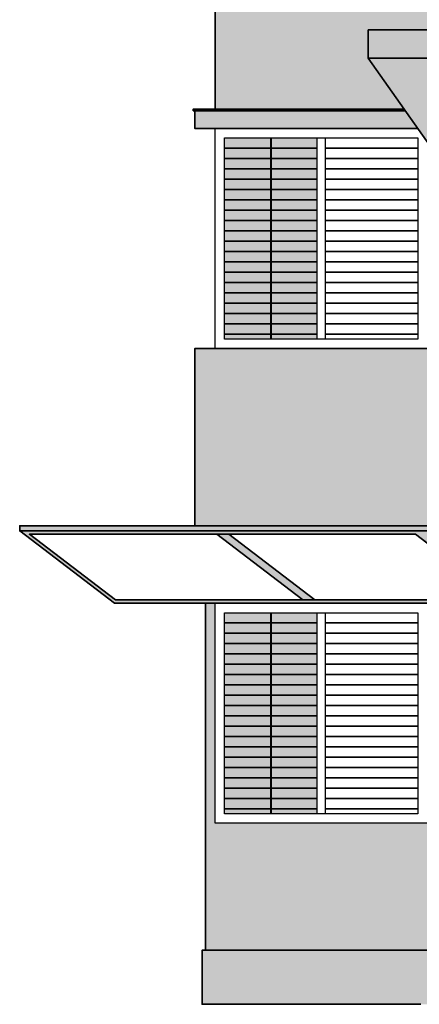
# Model space of a CAD drawing. Units: feet. Extents: x 2613 to 3913, y 950 to 1393.
# Tile 1 of 6: x 2613 to 2725, y 950 to 1226. Entities that reach past the tile are written whole.
import ezdxf

# ---------------------------------------------------------------- set-up
doc = ezdxf.new("R2010")
doc.units = ezdxf.units.FT
for name, color, linetype, lineweight in [('A-ELEV', 7, 'Continuous', 35), ('A-ELEV-PATT', 9, 'Continuous', 13), ('A-GLAZ', 4, 'Continuous', 25)]:
    doc.layers.add(name, color=color, linetype=linetype, lineweight=lineweight)

msp = doc.modelspace()

# ---------------------------------------------------------------- hatches: boundary and pattern name
at = {"layer": 'A-ELEV-PATT'}
h = msp.add_hatch(color=256, dxfattribs=at)
h.dxf.hatch_style = 1
h.paths.add_polyline_path([(3108.91, 1328.81), (3061.44, 1376.28), (2929.45, 1244.29), (2929.45, 1223.38), (2942.09, 1223.38), (2942.09, 1215.5), (2929.45, 1215.5), (2929.45, 1084.12), (3108.91, 1084.12), (3108.91, 1199.69), (3106.87, 1199.69), (3106.87, 1128.72), (3017.91, 1128.72), (3017.91, 1199.69), (3008.08, 1199.69), (3008.08, 1180.01), (3007.65, 1180.01), (3007.65, 1199.69), (3004.75, 1199.69), (3004.75, 1206.47), (3108.91, 1206.47)])
h.paths.add_polyline_path([(3061.44, 1376.28), (3193.8, 1243.92), (3193.8, 1233.84), (3204.34, 1246.9), (3061.54, 1389.71), (2918.82, 1247), (2929.45, 1233.69), (2929.45, 1244.29)])
h.paths.add_polyline_path([(3061.54, 1389.71), (3204.34, 1246.9), (3206.69, 1248.02), (3061.63, 1393.09), (2916.59, 1248.06), (2918.82, 1247)])
h.paths.add_polyline_path([(2925.65, 1257.12), (2667.59, 1257.12), (2651.33, 1257.12), (2651.33, 1252.28), (2920.82, 1252.28)])
h.paths.add_polyline_path([(2920.82, 1252.28), (2651.33, 1252.28, -0.144454), (2652.15, 1251.12), (2667.59, 1251.12), (2919.65, 1251.12)])
h.paths.add_polyline_path([(2918.82, 1247), (2916.59, 1248.06), (2919.65, 1251.12), (2667.59, 1251.12), (2652.15, 1251.12), (2667.59, 1229.14), (2667.59, 1233.69), (2929.45, 1233.69)])
h.paths.add_polyline_path([(2710.6, 1223.38), (2929.45, 1223.38), (2929.45, 1233.69), (2667.59, 1233.69), (2667.59, 1229.14), (2667.59, 1201.16), (2720.67, 1201.16), (2710.6, 1215.5)])
h.paths.add_polyline_path([(2942.09, 1223.38), (2710.6, 1223.38), (2710.6, 1215.5), (2921.48, 1215.5), (2942.09, 1215.5)])
h.paths.add_polyline_path([(2929.45, 1215.5), (2921.48, 1215.5), (2710.6, 1215.5), (2733.47, 1182.94), (2733.47, 1195.74), (2741.22, 1195.74), (2929.45, 1195.74)])
h.paths.add_polyline_path([(2721, 1200.68), (2661.89, 1200.68), (2661.89, 1195.74), (2724.47, 1195.74)])
h.paths.add_polyline_path([(2733.47, 1182.94), (2727.27, 1191.76), (2727.27, 1133.88), (2731.7, 1133.88), (2731.7, 1169.74), (2731.61, 1169.74), (2731.61, 1170.13), (2733.47, 1170.13)])
h.paths.add_polyline_path([(2929.45, 1183.04), (2741.22, 1183.04), (2741.22, 1170.13), (2743.07, 1170.13), (2743.07, 1169.74), (2743.07, 1112.32), (2759.57, 1112.32), (2759.57, 1167.82), (2763.7, 1167.82), (2763.7, 1112.32), (2781.75, 1112.32), (2781.75, 1167.82), (2785.87, 1167.82), (2785.87, 1112.32), (2803.92, 1112.32), (2803.92, 1167.82), (2808.05, 1167.82), (2808.05, 1112.32), (2826.09, 1112.32), (2826.09, 1167.82), (2830.22, 1167.82), (2830.22, 1112.32), (2875.17, 1112.32), (2875.17, 1171.49), (2929.45, 1171.49)])
h.paths.add_polyline_path([(2731.7, 1133.88), (2661.89, 1133.88), (2661.89, 1084.12), (2730.99, 1084.12), (2730.99, 1112.32), (2731.7, 1112.32)])
h.paths.add_polyline_path([(2929.45, 1112.32), (2730.99, 1112.32), (2730.99, 1084.12), (2929.45, 1084.12)])
h.paths.add_polyline_path([(2929.45, 1084.12), (2730.99, 1084.12), (2661.89, 1084.12), (2612.72, 1084.12), (2612.72, 1082.68), (2929.45, 1082.68)])
h.paths.add_polyline_path([(2929.45, 1082.68), (2612.72, 1082.68), (2639.32, 1062.44), (2733.47, 1062.44), (2733.47, 1063.35), (2639.62, 1063.35), (2615.43, 1081.77), (2723.91, 1081.77), (2739.71, 1069.74), (2741.22, 1069.74), (2725.42, 1081.77), (2929.45, 1081.77)])
h.paths.add_polyline_path([(2671.42, 1081.77), (2668.07, 1081.77), (2692.27, 1063.35), (2695.62, 1063.35)], flags=17)
h.paths.add_polyline_path([(2741.22, 1069.74), (2741.22, 1068.59), (2748.11, 1063.35), (2741.22, 1063.35), (2741.22, 1062.44), (2750.82, 1062.44)], flags=17)
h.paths.add_polyline_path([(2929.45, 1081.77), (2725.42, 1081.77), (2750.82, 1062.44), (2741.22, 1062.44), (2741.22, 1047.95), (2743.07, 1047.95), (2743.07, 1047.56), (2743.07, 967.97), (2875.17, 967.97), (2875.17, 1066.37), (2929.45, 1066.37)])
h.paths.add_polyline_path([(2778.55, 1066.37), (2806.94, 1066.37), (2806.94, 982.04), (2778.55, 982.04)], flags=16)
h.paths.add_polyline_path([(2778.55, 1064.05), (2806.94, 1064.05), (2806.94, 1063.39), (2778.55, 1063.39)], flags=16)
h.paths.add_polyline_path([(2778.55, 1061.07), (2806.94, 1061.07), (2806.94, 1060.41), (2778.55, 1060.41)], flags=0)
h.paths.add_polyline_path([(2778.55, 1058.09), (2806.94, 1058.09), (2806.94, 1057.43), (2778.55, 1057.43)], flags=0)
h.paths.add_polyline_path([(2778.55, 1055.11), (2806.94, 1055.11), (2806.94, 1054.45), (2778.55, 1054.45)], flags=0)
h.paths.add_polyline_path([(2778.55, 1052.13), (2806.94, 1052.13), (2806.94, 1051.47), (2778.55, 1051.47)], flags=0)
h.paths.add_polyline_path([(2778.55, 1049.15), (2806.94, 1049.15), (2806.94, 1048.49), (2778.55, 1048.49)], flags=0)
h.paths.add_polyline_path([(2778.55, 1046.18), (2806.94, 1046.18), (2806.94, 1045.51), (2778.55, 1045.51)], flags=0)
h.paths.add_polyline_path([(2778.55, 1043.2), (2806.94, 1043.2), (2806.94, 1042.53), (2778.55, 1042.53)], flags=0)
h.paths.add_polyline_path([(2778.55, 1040.22), (2806.94, 1040.22), (2806.94, 1039.56), (2778.55, 1039.56)], flags=0)
h.paths.add_polyline_path([(2778.55, 1037.24), (2806.94, 1037.24), (2806.94, 1036.58), (2778.55, 1036.58)], flags=0)
h.paths.add_polyline_path([(2778.55, 1034.26), (2806.94, 1034.26), (2806.94, 1033.6), (2778.55, 1033.6)], flags=0)
h.paths.add_polyline_path([(2778.55, 1031.28), (2806.94, 1031.28), (2806.94, 1030.62), (2778.55, 1030.62)], flags=0)
h.paths.add_polyline_path([(2778.55, 1028.3), (2806.94, 1028.3), (2806.94, 1027.64), (2778.55, 1027.64)], flags=0)
h.paths.add_polyline_path([(2778.55, 1025.32), (2806.94, 1025.32), (2806.94, 1024.66), (2778.55, 1024.66)], flags=0)
h.paths.add_polyline_path([(2778.55, 1022.34), (2806.94, 1022.34), (2806.94, 1021.68), (2778.55, 1021.68)], flags=0)
h.paths.add_polyline_path([(2778.55, 1019.36), (2806.94, 1019.36), (2806.94, 1018.7), (2778.55, 1018.7)], flags=0)
h.paths.add_polyline_path([(2778.55, 1016.71), (2806.94, 1016.71), (2806.94, 1016.05), (2778.55, 1016.05)], flags=0)
h.paths.add_polyline_path([(2824.02, 1066.37), (2852.41, 1066.37), (2852.41, 982.04), (2824.02, 982.04)], flags=16)
h.paths.add_polyline_path([(2778.55, 1014.07), (2806.94, 1014.07), (2806.94, 1013.4), (2778.55, 1013.4)], flags=0)
h.paths.add_polyline_path([(2824.02, 1064.05), (2852.41, 1064.05), (2852.41, 1063.39), (2824.02, 1063.39)], flags=16)
h.paths.add_polyline_path([(2824.02, 1061.07), (2852.41, 1061.07), (2852.41, 1060.41), (2824.02, 1060.41)], flags=0)
h.paths.add_polyline_path([(2824.02, 1058.09), (2852.41, 1058.09), (2852.41, 1057.43), (2824.02, 1057.43)], flags=0)
h.paths.add_polyline_path([(2824.02, 1055.11), (2852.41, 1055.11), (2852.41, 1054.45), (2824.02, 1054.45)], flags=16)
h.paths.add_polyline_path([(2824.02, 1052.13), (2852.41, 1052.13), (2852.41, 1051.47), (2824.02, 1051.47)], flags=0)
h.paths.add_polyline_path([(2778.55, 1011.09), (2806.94, 1011.09), (2806.94, 1010.43), (2778.55, 1010.43)], flags=0)
h.paths.add_polyline_path([(2824.02, 1049.15), (2852.41, 1049.15), (2852.41, 1048.49), (2824.02, 1048.49)], flags=0)
h.paths.add_polyline_path([(2824.02, 1046.18), (2852.41, 1046.18), (2852.41, 1045.51), (2824.02, 1045.51)], flags=0)
h.paths.add_polyline_path([(2824.02, 1043.2), (2852.41, 1043.2), (2852.41, 1042.53), (2824.02, 1042.53)], flags=0)
h.paths.add_polyline_path([(2778.55, 1008.11), (2806.94, 1008.11), (2806.94, 1007.45), (2778.55, 1007.45)], flags=0)
h.paths.add_polyline_path([(2824.02, 1040.22), (2852.41, 1040.22), (2852.41, 1039.56), (2824.02, 1039.56)], flags=0)
h.paths.add_polyline_path([(2824.02, 1037.24), (2852.41, 1037.24), (2852.41, 1036.58), (2824.02, 1036.58)], flags=0)
h.paths.add_polyline_path([(2778.55, 1005.13), (2806.94, 1005.13), (2806.94, 1004.47), (2778.55, 1004.47)], flags=0)
h.paths.add_polyline_path([(2824.02, 1034.26), (2852.41, 1034.26), (2852.41, 1033.6), (2824.02, 1033.6)], flags=0)
h.paths.add_polyline_path([(2824.02, 1031.28), (2852.41, 1031.28), (2852.41, 1030.62), (2824.02, 1030.62)], flags=0)
h.paths.add_polyline_path([(2778.55, 1002.15), (2806.94, 1002.15), (2806.94, 1001.49), (2778.55, 1001.49)], flags=0)
h.paths.add_polyline_path([(2824.02, 1028.3), (2852.41, 1028.3), (2852.41, 1027.64), (2824.02, 1027.64)], flags=0)
h.paths.add_polyline_path([(2778.55, 999.17), (2806.94, 999.17), (2806.94, 998.51), (2778.55, 998.51)], flags=0)
h.paths.add_polyline_path([(2824.02, 1025.32), (2852.41, 1025.32), (2852.41, 1024.66), (2824.02, 1024.66)], flags=0)
h.paths.add_polyline_path([(2824.02, 1022.34), (2852.41, 1022.34), (2852.41, 1021.68), (2824.02, 1021.68)], flags=0)
h.paths.add_polyline_path([(2778.55, 996.19), (2806.94, 996.19), (2806.94, 995.53), (2778.55, 995.53)], flags=0)
h.paths.add_polyline_path([(2824.02, 1019.36), (2852.41, 1019.36), (2852.41, 1018.7), (2824.02, 1018.7)], flags=0)
h.paths.add_polyline_path([(2778.55, 993.21), (2806.94, 993.21), (2806.94, 992.55), (2778.55, 992.55)], flags=0)
h.paths.add_polyline_path([(2824.02, 1016.38), (2852.41, 1016.38), (2852.41, 1015.72), (2824.02, 1015.72)], flags=0)
h.paths.add_polyline_path([(2824.02, 1013.4), (2852.41, 1013.4), (2852.41, 1012.74), (2824.02, 1012.74)], flags=0)
h.paths.add_polyline_path([(2778.55, 990.23), (2806.94, 990.23), (2806.94, 989.57), (2778.55, 989.57)], flags=0)
h.paths.add_polyline_path([(2824.02, 1010.43), (2852.41, 1010.43), (2852.41, 1009.76), (2824.02, 1009.76)], flags=0)
h.paths.add_polyline_path([(2778.55, 987.25), (2806.94, 987.25), (2806.94, 986.59), (2778.55, 986.59)], flags=0)
h.paths.add_polyline_path([(2824.02, 1007.45), (2852.41, 1007.45), (2852.41, 1006.78), (2824.02, 1006.78)], flags=0)
h.paths.add_polyline_path([(2778.55, 984.27), (2806.94, 984.27), (2806.94, 983.61), (2778.55, 983.61)], flags=0)
h.paths.add_polyline_path([(2824.02, 1004.47), (2852.41, 1004.47), (2852.41, 1003.81), (2824.02, 1003.81)], flags=0)
h.paths.add_polyline_path([(2824.02, 1001.49), (2852.41, 1001.49), (2852.41, 1000.83), (2824.02, 1000.83)], flags=0)
h.paths.add_polyline_path([(2824.02, 998.51), (2852.41, 998.51), (2852.41, 997.85), (2824.02, 997.85)], flags=0)
h.paths.add_polyline_path([(2824.02, 995.53), (2852.41, 995.53), (2852.41, 994.87), (2824.02, 994.87)], flags=0)
h.paths.add_polyline_path([(2824.02, 992.55), (2852.41, 992.55), (2852.41, 991.89), (2824.02, 991.89)], flags=0)
h.paths.add_polyline_path([(2824.02, 989.57), (2852.41, 989.57), (2852.41, 988.91), (2824.02, 988.91)], flags=0)
h.paths.add_polyline_path([(2824.02, 986.59), (2852.41, 986.59), (2852.41, 985.93), (2824.02, 985.93)], flags=0)
h.paths.add_polyline_path([(2824.02, 983.61), (2852.41, 983.61), (2852.41, 982.95), (2824.02, 982.95)], flags=0)
h.paths.add_polyline_path([(2731.7, 1047.56), (2731.61, 1047.56), (2731.61, 1047.95), (2733.47, 1047.95), (2733.47, 1062.44), (2727.27, 1062.44), (2727.27, 1000.58), (2667.59, 1000.58), (2667.59, 1062.44), (2664.87, 1062.44), (2664.87, 965.01), (2730.76, 964.93), (2730.76, 967.97), (2731.7, 967.97)])
h.paths.add_polyline_path([(2728.06, 961.9), (2730.76, 961.9), (2730.76, 964.93), (2663.94, 964.93), (2663.94, 949.74), (2725.36, 949.74), (2725.36, 955.82), (2728.06, 955.82)])
h.paths.add_polyline_path([(2929.45, 967.97), (2730.76, 967.97), (2730.76, 961.9), (2929.45, 961.9)])
h.paths.add_polyline_path([(2929.45, 961.9), (2730.76, 961.9), (2728.06, 961.9), (2728.06, 955.82), (2929.45, 955.82)])
h.paths.add_polyline_path([(2929.45, 955.82), (2728.06, 955.82), (2725.36, 955.82), (2725.36, 949.74), (2929.45, 949.74)])
h.paths.add_polyline_path([(2741.22, 1069.74), (2733.47, 1069.74), (2733.47, 1047.95), (2741.22, 1047.95)], flags=17)
h.paths.add_polyline_path([(2741.22, 1195.74), (2733.47, 1195.74), (2733.47, 1182.94), (2733.47, 1170.13), (2741.22, 1170.13), (2741.22, 1183.04)])
h.paths.add_polyline_path([(3193.8, 1084.12), (2929.45, 1084.12), (2929.45, 1082.68), (2929.45, 1081.77), (2929.45, 1066.37), (2929.45, 949.74), (3193.8, 949.74)])
h.paths.add_polyline_path([(2937.79, 1075.78), (3185.46, 1075.78), (3185.46, 958.09), (2937.79, 958.09)], flags=16)
h.paths.add_polyline_path([(3011.76, 1075.78), (3104.46, 1075.78), (3104.46, 993.6), (3011.76, 993.6)], flags=0)
h.paths.add_polyline_path([(3015.24, 1075.78), (3016.57, 1075.78), (3016.57, 1060.85), (3043.1, 1060.85), (3043.1, 1075.78), (3045.77, 1075.78), (3045.77, 997.08), (3070.45, 997.08), (3070.45, 1075.78), (3073.12, 1075.78), (3073.12, 1060.85), (3099.64, 1060.85), (3099.64, 1075.78), (3100.98, 1075.78), (3100.98, 997.08), (3099.64, 997.08), (3015.24, 997.08)], flags=0)
h = msp.add_hatch(color=256, dxfattribs=at)
h.dxf.hatch_style = 1
h.paths.add_polyline_path([(2768.1, 1195.09), (2741.95, 1195.09), (2741.95, 1183.7), (2768.1, 1183.7)])
h.paths.add_polyline_path([(2794.91, 1195.09), (2768.76, 1195.09), (2768.76, 1183.7), (2794.91, 1183.7)])
h.paths.add_polyline_path([(2821.72, 1195.09), (2795.57, 1195.09), (2795.57, 1183.7), (2821.72, 1183.7)])
h.paths.add_polyline_path([(2848.53, 1195.09), (2822.38, 1195.09), (2822.38, 1183.7), (2848.53, 1183.7)])
h.paths.add_polyline_path([(2875.34, 1195.09), (2849.19, 1195.09), (2849.19, 1183.7), (2875.34, 1183.7)])
h.paths.add_polyline_path([(2683.29, 1193.04), (2670.29, 1193.04), (2670.29, 1190.17), (2683.29, 1190.17)])
h.paths.add_polyline_path([(2696.31, 1193.04), (2683.32, 1193.04), (2683.32, 1190.17), (2696.31, 1190.17)])
h.paths.add_polyline_path([(2696.31, 1190.14), (2683.32, 1190.14), (2683.32, 1187.27), (2696.31, 1187.27)])
h.paths.add_polyline_path([(2683.29, 1190.14), (2670.29, 1190.14), (2670.29, 1187.27), (2683.29, 1187.27)])
h.paths.add_polyline_path([(2683.29, 1187.24), (2670.29, 1187.24), (2670.29, 1184.37), (2683.29, 1184.37)])
h.paths.add_polyline_path([(2696.31, 1187.24), (2683.32, 1187.24), (2683.32, 1184.37), (2696.31, 1184.37)])
h.paths.add_polyline_path([(2683.29, 1184.34), (2670.29, 1184.34), (2670.29, 1181.47), (2683.29, 1181.47)])
h.paths.add_polyline_path([(2696.31, 1184.34), (2683.32, 1184.34), (2683.32, 1181.47), (2696.31, 1181.47)])
h.paths.add_polyline_path([(2683.29, 1181.44), (2670.29, 1181.44), (2670.29, 1178.57), (2683.29, 1178.57)])
h.paths.add_polyline_path([(2696.31, 1181.44), (2683.32, 1181.44), (2683.32, 1178.57), (2696.31, 1178.57)])
h.paths.add_polyline_path([(2696.31, 1178.53), (2683.32, 1178.53), (2683.32, 1175.67), (2696.31, 1175.67)])
h.paths.add_polyline_path([(2683.29, 1178.53), (2670.29, 1178.53), (2670.29, 1175.67), (2683.29, 1175.67)])
h.paths.add_polyline_path([(2683.29, 1175.63), (2670.29, 1175.63), (2670.29, 1172.76), (2683.29, 1172.76)])
h.paths.add_polyline_path([(2696.31, 1175.63), (2683.32, 1175.63), (2683.32, 1172.76), (2696.31, 1172.76)])
h.paths.add_polyline_path([(2683.29, 1172.73), (2670.29, 1172.73), (2670.29, 1169.86), (2683.29, 1169.86)])
h.paths.add_polyline_path([(2696.31, 1172.73), (2683.32, 1172.73), (2683.32, 1169.86), (2696.31, 1169.86)])
h.paths.add_polyline_path([(2696.31, 1169.83), (2683.32, 1169.83), (2683.32, 1166.96), (2696.31, 1166.96)])
h.paths.add_polyline_path([(2683.29, 1169.83), (2670.29, 1169.83), (2670.29, 1166.96), (2683.29, 1166.96)])
h.paths.add_polyline_path([(2696.31, 1166.93), (2683.32, 1166.93), (2683.32, 1164.06), (2696.31, 1164.06)])
h.paths.add_polyline_path([(2683.29, 1166.93), (2670.29, 1166.93), (2670.29, 1164.06), (2683.29, 1164.06)])
h.paths.add_polyline_path([(2683.29, 1164.03), (2670.29, 1164.03), (2670.29, 1161.16), (2683.29, 1161.16)])
h.paths.add_polyline_path([(2696.31, 1164.03), (2683.32, 1164.03), (2683.32, 1161.16), (2696.31, 1161.16)])
h.paths.add_polyline_path([(2696.31, 1161.12), (2683.32, 1161.12), (2683.32, 1158.25), (2696.31, 1158.25)])
h.paths.add_polyline_path([(2683.29, 1161.12), (2670.29, 1161.12), (2670.29, 1158.25), (2683.29, 1158.25)])
h.paths.add_polyline_path([(2683.29, 1158.22), (2670.29, 1158.22), (2670.29, 1155.35), (2683.29, 1155.35)])
h.paths.add_polyline_path([(2696.31, 1158.22), (2683.32, 1158.22), (2683.32, 1155.35), (2696.31, 1155.35)])
h.paths.add_polyline_path([(2696.31, 1155.32), (2683.32, 1155.32), (2683.32, 1152.45), (2696.31, 1152.45)])
h.paths.add_polyline_path([(2683.29, 1155.32), (2670.29, 1155.32), (2670.29, 1152.45), (2683.29, 1152.45)])
h.paths.add_polyline_path([(2683.29, 1152.42), (2670.29, 1152.42), (2670.29, 1149.55), (2683.29, 1149.55)])
h.paths.add_polyline_path([(2696.31, 1152.42), (2683.32, 1152.42), (2683.32, 1149.55), (2696.31, 1149.55)])
h.paths.add_polyline_path([(2683.29, 1149.52), (2670.29, 1149.52), (2670.29, 1146.65), (2683.29, 1146.65)])
h.paths.add_polyline_path([(2696.31, 1149.52), (2683.32, 1149.52), (2683.32, 1146.65), (2696.31, 1146.65)])
h.paths.add_polyline_path([(2696.31, 1146.61), (2683.32, 1146.61), (2683.32, 1143.75), (2696.31, 1143.75)])
h.paths.add_polyline_path([(2683.29, 1146.61), (2670.29, 1146.61), (2670.29, 1143.75), (2683.29, 1143.75)])
h.paths.add_polyline_path([(2683.29, 1143.71), (2670.29, 1143.71), (2670.29, 1140.84), (2683.29, 1140.84)])
h.paths.add_polyline_path([(2696.31, 1143.71), (2683.32, 1143.71), (2683.32, 1140.84), (2696.31, 1140.84)])
h.paths.add_polyline_path([(2683.29, 1140.81), (2670.29, 1140.81), (2670.29, 1137.94), (2683.29, 1137.94)])
h.paths.add_polyline_path([(2696.31, 1140.81), (2683.32, 1140.81), (2683.32, 1137.94), (2696.31, 1137.94)])
h.paths.add_polyline_path([(2683.29, 1137.91), (2670.29, 1137.91), (2670.29, 1136.58), (2683.29, 1136.58)])
h.paths.add_polyline_path([(2696.31, 1137.91), (2683.32, 1137.91), (2683.32, 1136.58), (2696.31, 1136.58)])
h.paths.add_polyline_path([(3074.7, 1198.4), (3050.02, 1198.4), (3050.02, 1130.01), (3074.7, 1130.01)])
h.paths.add_polyline_path([(3047.34, 1198.4), (3019.29, 1198.4), (3019.29, 1184.76), (3047.34, 1184.76)])
h.paths.add_polyline_path([(3047.34, 1183.78), (3019.29, 1183.78), (3019.29, 1130.01), (3047.34, 1130.01)])
h.paths.add_polyline_path([(3105.48, 1198.4), (3077.37, 1198.4), (3077.37, 1184.76), (3105.48, 1184.76)])
h.paths.add_polyline_path([(3105.48, 1183.78), (3077.37, 1183.78), (3077.37, 1130.01), (3105.48, 1130.01)])
h.paths.add_polyline_path([(3070.45, 1075.78), (3045.77, 1075.78), (3045.77, 997.08), (3070.45, 997.08)])
h.paths.add_polyline_path([(3099.64, 1075.78), (3073.12, 1075.78), (3073.12, 1060.85), (3099.64, 1060.85)])
h.paths.add_polyline_path([(3099.64, 1059.87), (3073.12, 1059.87), (3073.12, 997.08), (3099.64, 997.08)])
h.paths.add_polyline_path([(3043.1, 1075.78), (3016.57, 1075.78), (3016.57, 1060.85), (3043.1, 1060.85)])
h.paths.add_polyline_path([(3043.1, 1059.87), (3016.57, 1059.87), (3016.57, 997.08), (3043.1, 997.08)])
h.paths.add_polyline_path([(2683.29, 1059.73), (2670.29, 1059.73), (2670.29, 1056.87), (2683.29, 1056.87)])
h.paths.add_polyline_path([(2696.31, 1059.73), (2683.32, 1059.73), (2683.32, 1056.87), (2696.31, 1056.87)])
h.paths.add_polyline_path([(2696.31, 1056.83), (2683.32, 1056.83), (2683.32, 1053.96), (2696.31, 1053.96)])
h.paths.add_polyline_path([(2683.29, 1056.83), (2670.29, 1056.83), (2670.29, 1053.96), (2683.29, 1053.96)])
h.paths.add_polyline_path([(2683.29, 1053.93), (2670.29, 1053.93), (2670.29, 1051.06), (2683.29, 1051.06)])
h.paths.add_polyline_path([(2696.31, 1053.93), (2683.32, 1053.93), (2683.32, 1051.06), (2696.31, 1051.06)])
h.paths.add_polyline_path([(2683.29, 1051.03), (2670.29, 1051.03), (2670.29, 1048.16), (2683.29, 1048.16)])
h.paths.add_polyline_path([(2696.31, 1051.03), (2683.32, 1051.03), (2683.32, 1048.16), (2696.31, 1048.16)])
h.paths.add_polyline_path([(2683.29, 1048.13), (2670.29, 1048.13), (2670.29, 1045.26), (2683.29, 1045.26)])
h.paths.add_polyline_path([(2696.31, 1048.13), (2683.32, 1048.13), (2683.32, 1045.26), (2696.31, 1045.26)])
h.paths.add_polyline_path([(2696.31, 1045.23), (2683.32, 1045.23), (2683.32, 1042.36), (2696.31, 1042.36)])
h.paths.add_polyline_path([(2683.29, 1045.23), (2670.29, 1045.23), (2670.29, 1042.36), (2683.29, 1042.36)])
h.paths.add_polyline_path([(2683.29, 1042.32), (2670.29, 1042.32), (2670.29, 1039.46), (2683.29, 1039.46)])
h.paths.add_polyline_path([(2696.31, 1042.32), (2683.32, 1042.32), (2683.32, 1039.46), (2696.31, 1039.46)])
h.paths.add_polyline_path([(2696.31, 1039.42), (2683.32, 1039.42), (2683.32, 1036.55), (2696.31, 1036.55)])
h.paths.add_polyline_path([(2683.29, 1039.42), (2670.29, 1039.42), (2670.29, 1036.55), (2683.29, 1036.55)])
h.paths.add_polyline_path([(2683.29, 1036.52), (2670.29, 1036.52), (2670.29, 1033.65), (2683.29, 1033.65)])
h.paths.add_polyline_path([(2696.31, 1036.52), (2683.32, 1036.52), (2683.32, 1033.65), (2696.31, 1033.65)])
h.paths.add_polyline_path([(2696.31, 1033.62), (2683.32, 1033.62), (2683.32, 1030.75), (2696.31, 1030.75)])
h.paths.add_polyline_path([(2683.29, 1033.62), (2670.29, 1033.62), (2670.29, 1030.75), (2683.29, 1030.75)])
h.paths.add_polyline_path([(2696.31, 1030.72), (2683.32, 1030.72), (2683.32, 1027.85), (2696.31, 1027.85)])
h.paths.add_polyline_path([(2683.29, 1030.72), (2670.29, 1030.72), (2670.29, 1027.85), (2683.29, 1027.85)])
h.paths.add_polyline_path([(2683.29, 1027.82), (2670.29, 1027.82), (2670.29, 1024.95), (2683.29, 1024.95)])
h.paths.add_polyline_path([(2696.31, 1027.82), (2683.32, 1027.82), (2683.32, 1024.95), (2696.31, 1024.95)])
h.paths.add_polyline_path([(2696.31, 1024.91), (2683.32, 1024.91), (2683.32, 1022.05), (2696.31, 1022.05)])
h.paths.add_polyline_path([(2683.29, 1024.91), (2670.29, 1024.91), (2670.29, 1022.05), (2683.29, 1022.05)])
h.paths.add_polyline_path([(2683.29, 1022.01), (2670.29, 1022.01), (2670.29, 1019.14), (2683.29, 1019.14)])
h.paths.add_polyline_path([(2696.31, 1022.01), (2683.32, 1022.01), (2683.32, 1019.14), (2696.31, 1019.14)])
h.paths.add_polyline_path([(2696.31, 1019.11), (2683.32, 1019.11), (2683.32, 1016.24), (2696.31, 1016.24)])
h.paths.add_polyline_path([(2683.29, 1019.11), (2670.29, 1019.11), (2670.29, 1016.24), (2683.29, 1016.24)])
h.paths.add_polyline_path([(2683.29, 1016.21), (2670.29, 1016.21), (2670.29, 1013.34), (2683.29, 1013.34)])
h.paths.add_polyline_path([(2696.31, 1016.21), (2683.32, 1016.21), (2683.32, 1013.34), (2696.31, 1013.34)])
h.paths.add_polyline_path([(2696.31, 1013.31), (2683.32, 1013.31), (2683.32, 1010.44), (2696.31, 1010.44)])
h.paths.add_polyline_path([(2683.29, 1013.31), (2670.29, 1013.31), (2670.29, 1010.44), (2683.29, 1010.44)])
h.paths.add_polyline_path([(2683.29, 1010.41), (2670.29, 1010.41), (2670.29, 1007.54), (2683.29, 1007.54)])
h.paths.add_polyline_path([(2696.31, 1010.41), (2683.32, 1010.41), (2683.32, 1007.54), (2696.31, 1007.54)])
h.paths.add_polyline_path([(2696.31, 1007.5), (2683.32, 1007.5), (2683.32, 1004.64), (2696.31, 1004.64)])
h.paths.add_polyline_path([(2683.29, 1007.5), (2670.29, 1007.5), (2670.29, 1004.64), (2683.29, 1004.64)])
h.paths.add_polyline_path([(2683.29, 1004.6), (2670.29, 1004.6), (2670.29, 1003.28), (2683.29, 1003.28)])
h.paths.add_polyline_path([(2696.31, 1004.6), (2683.32, 1004.6), (2683.32, 1003.28), (2696.31, 1003.28)])
h.paths.add_polyline_path([(2806.94, 1066.37), (2778.55, 1066.37), (2778.55, 1064.05), (2806.94, 1064.05)])
h.paths.add_polyline_path([(2806.94, 1063.39), (2778.55, 1063.39), (2778.55, 1061.07), (2806.94, 1061.07)])
h.paths.add_polyline_path([(2806.94, 1060.41), (2778.55, 1060.41), (2778.55, 1058.09), (2806.94, 1058.09)])
h.paths.add_polyline_path([(2806.94, 1057.43), (2778.55, 1057.43), (2778.55, 1055.11), (2806.94, 1055.11)])
h.paths.add_polyline_path([(2806.94, 1054.45), (2778.55, 1054.45), (2778.55, 1052.13), (2806.94, 1052.13)])
h.paths.add_polyline_path([(2806.94, 1051.47), (2778.55, 1051.47), (2778.55, 1049.15), (2806.94, 1049.15)])
h.paths.add_polyline_path([(2806.94, 1048.49), (2778.55, 1048.49), (2778.55, 1046.18), (2806.94, 1046.18)])
h.paths.add_polyline_path([(2806.94, 1045.51), (2778.55, 1045.51), (2778.55, 1043.2), (2806.94, 1043.2)])
h.paths.add_polyline_path([(2806.94, 1042.53), (2778.55, 1042.53), (2778.55, 1040.22), (2806.94, 1040.22)])
h.paths.add_polyline_path([(2806.94, 1039.56), (2778.55, 1039.56), (2778.55, 1037.24), (2806.94, 1037.24)])
h.paths.add_polyline_path([(2806.94, 1036.58), (2778.55, 1036.58), (2778.55, 1034.26), (2806.94, 1034.26)])
h.paths.add_polyline_path([(2806.94, 1033.6), (2778.55, 1033.6), (2778.55, 1031.28), (2806.94, 1031.28)])
h.paths.add_polyline_path([(2806.94, 1030.62), (2778.55, 1030.62), (2778.55, 1028.3), (2806.94, 1028.3)])
h.paths.add_polyline_path([(2806.94, 1027.64), (2778.55, 1027.64), (2778.55, 1025.32), (2806.94, 1025.32)])
h.paths.add_polyline_path([(2806.94, 1024.66), (2778.55, 1024.66), (2778.55, 1022.34), (2806.94, 1022.34)])
h.paths.add_polyline_path([(2806.94, 1021.68), (2778.55, 1021.68), (2778.55, 1019.36), (2806.94, 1019.36)])
h.paths.add_polyline_path([(2806.94, 1018.7), (2778.55, 1018.7), (2778.55, 1016.71), (2806.94, 1016.71)])
h.paths.add_polyline_path([(2806.94, 1016.05), (2778.55, 1016.05), (2778.55, 1014.07), (2806.94, 1014.07)])
h.paths.add_polyline_path([(2806.94, 1013.4), (2778.55, 1013.4), (2778.55, 1011.09), (2806.94, 1011.09)])
h.paths.add_polyline_path([(2806.94, 1010.43), (2778.55, 1010.43), (2778.55, 1008.11), (2806.94, 1008.11)])
h.paths.add_polyline_path([(2806.94, 1007.45), (2778.55, 1007.45), (2778.55, 1005.13), (2806.94, 1005.13)])
h.paths.add_polyline_path([(2806.94, 1004.47), (2778.55, 1004.47), (2778.55, 1002.15), (2806.94, 1002.15)])
h.paths.add_polyline_path([(2806.94, 1001.49), (2778.55, 1001.49), (2778.55, 999.17), (2806.94, 999.17)])
h.paths.add_polyline_path([(2806.94, 998.51), (2778.55, 998.51), (2778.55, 996.19), (2806.94, 996.19)])
h.paths.add_polyline_path([(2806.94, 983.61), (2778.55, 983.61), (2778.55, 982.04), (2806.94, 982.04)])
h.paths.add_polyline_path([(2806.94, 986.59), (2778.55, 986.59), (2778.55, 984.27), (2806.94, 984.27)])
h.paths.add_polyline_path([(2806.94, 989.57), (2778.55, 989.57), (2778.55, 987.25), (2806.94, 987.25)])
h.paths.add_polyline_path([(2806.94, 992.55), (2778.55, 992.55), (2778.55, 990.23), (2806.94, 990.23)])
h.paths.add_polyline_path([(2806.94, 995.53), (2778.55, 995.53), (2778.55, 993.21), (2806.94, 993.21)])
h.paths.add_polyline_path([(2852.41, 985.93), (2824.02, 985.93), (2824.02, 983.61), (2852.41, 983.61)])
h.paths.add_polyline_path([(2852.41, 982.95), (2824.02, 982.95), (2824.02, 982.04), (2852.41, 982.04)])
h.paths.add_polyline_path([(2852.41, 988.91), (2824.02, 988.91), (2824.02, 986.59), (2852.41, 986.59)])
h.paths.add_polyline_path([(2852.41, 991.89), (2824.02, 991.89), (2824.02, 989.57), (2852.41, 989.57)])
h.paths.add_polyline_path([(2852.41, 994.87), (2824.02, 994.87), (2824.02, 992.55), (2852.41, 992.55)])
h.paths.add_polyline_path([(2852.41, 997.85), (2824.02, 997.85), (2824.02, 995.53), (2852.41, 995.53)])
h.paths.add_polyline_path([(2852.41, 1000.83), (2824.02, 1000.83), (2824.02, 998.51), (2852.41, 998.51)])
h.paths.add_polyline_path([(2852.41, 1003.81), (2824.02, 1003.81), (2824.02, 1001.49), (2852.41, 1001.49)])
h.paths.add_polyline_path([(2852.41, 1006.78), (2824.02, 1006.78), (2824.02, 1004.47), (2852.41, 1004.47)])
h.paths.add_polyline_path([(2852.41, 1009.76), (2824.02, 1009.76), (2824.02, 1007.45), (2852.41, 1007.45)])
h.paths.add_polyline_path([(2852.41, 1012.74), (2824.02, 1012.74), (2824.02, 1010.43), (2852.41, 1010.43)])
h.paths.add_polyline_path([(2852.41, 1015.72), (2824.02, 1015.72), (2824.02, 1013.4), (2852.41, 1013.4)])
h.paths.add_polyline_path([(2852.41, 1018.7), (2824.02, 1018.7), (2824.02, 1016.38), (2852.41, 1016.38)])
h.paths.add_polyline_path([(2852.41, 1021.68), (2824.02, 1021.68), (2824.02, 1019.36), (2852.41, 1019.36)])
h.paths.add_polyline_path([(2852.41, 1024.66), (2824.02, 1024.66), (2824.02, 1022.34), (2852.41, 1022.34)])
h.paths.add_polyline_path([(2852.41, 1027.64), (2824.02, 1027.64), (2824.02, 1025.32), (2852.41, 1025.32)])
h.paths.add_polyline_path([(2852.41, 1030.62), (2824.02, 1030.62), (2824.02, 1028.3), (2852.41, 1028.3)])
h.paths.add_polyline_path([(2852.41, 1033.6), (2824.02, 1033.6), (2824.02, 1031.28), (2852.41, 1031.28)])
h.paths.add_polyline_path([(2852.41, 1036.58), (2824.02, 1036.58), (2824.02, 1034.26), (2852.41, 1034.26)])
h.paths.add_polyline_path([(2852.41, 1039.56), (2824.02, 1039.56), (2824.02, 1037.24), (2852.41, 1037.24)])
h.paths.add_polyline_path([(2852.41, 1042.53), (2824.02, 1042.53), (2824.02, 1040.22), (2852.41, 1040.22)])
h.paths.add_polyline_path([(2852.41, 1045.51), (2824.02, 1045.51), (2824.02, 1043.2), (2852.41, 1043.2)])
h.paths.add_polyline_path([(2852.41, 1048.49), (2824.02, 1048.49), (2824.02, 1046.18), (2852.41, 1046.18)])
h.paths.add_polyline_path([(2852.41, 1066.37), (2824.02, 1066.37), (2824.02, 1049.15), (2852.41, 1049.15)])

# ---------------------------------------------------------------- linework, layer by layer
at = {"layer": 'A-ELEV'}
for p, q in [((2942.09, 1223.38), (2710.6, 1223.38)), ((2710.6, 1215.5), (2710.6, 1223.38)), ((2942.09, 1223.38), (2710.6, 1223.38)), ((2710.6, 1215.5), (2710.6, 1223.38)), ((2733.47, 1182.94), (2710.6, 1215.5)), ((2710.6, 1215.5), (2921.48, 1215.5)), ((2733.47, 1182.94), (2710.6, 1215.5)), ((2710.6, 1215.5), (2921.48, 1215.5)), ((2661.89, 1195.74), (2667.59, 1195.74)), ((2661.89, 1195.74), (2667.59, 1195.74)), ((2615.43, 1081.77), (2639.62, 1063.35)), ((2615.43, 1081.77), (2639.62, 1063.35)), ((2668.07, 1081.77), (2692.27, 1063.35)), ((2668.07, 1081.77), (2692.27, 1063.35)), ((2671.42, 1081.77), (2695.62, 1063.35)), ((2671.42, 1081.77), (2695.62, 1063.35)), ((2664.87, 1062.44), (2664.87, 965.01)), ((2664.87, 1062.44), (2664.87, 965.01)), ((2664.87, 965.01), (2730.76, 964.93)), ((2664.87, 965.01), (2730.76, 964.93))]:
    msp.add_line(p, q, dxfattribs=at)
for points in [[(2929.45, 1233.69), (2667.59, 1233.69), (2667.59, 1229.14), (2667.59, 1201.16)], [(2929.45, 1233.69), (2667.59, 1233.69), (2667.59, 1229.14), (2667.59, 1201.16)], [(2721, 1200.68), (2661.49, 1200.68), (2661.49, 1201.16), (2720.67, 1201.16)], [(2721, 1200.68), (2661.49, 1200.68), (2661.49, 1201.16), (2720.67, 1201.16)], [(2721, 1200.68), (2661.89, 1200.68), (2661.89, 1195.74), (2724.47, 1195.74)], [(2721, 1200.68), (2661.89, 1200.68), (2661.89, 1195.74), (2724.47, 1195.74)], [(2730.99, 1091.48), (2730.99, 1084.12), (2661.89, 1084.12), (2661.89, 1133.88), (2731.7, 1133.88)], [(2730.99, 1091.48), (2730.99, 1084.12), (2661.89, 1084.12), (2661.89, 1133.88), (2731.7, 1133.88)], [(2929.45, 1082.68), (2612.72, 1082.68), (2639.32, 1062.44), (2733.47, 1062.44)], [(2929.45, 1082.68), (2612.72, 1082.68), (2639.32, 1062.44), (2733.47, 1062.44)], [(2739.71, 1069.74), (2723.91, 1081.77), (2615.43, 1081.77), (2639.62, 1063.35), (2733.47, 1063.35)], [(2733.47, 1074.5), (2723.91, 1081.77), (2615.43, 1081.77), (2639.62, 1063.35), (2733.47, 1063.35)], [(2730.76, 964.93), (2663.94, 964.93), (2663.94, 949.74), (2725.36, 949.74)], [(2730.76, 964.93), (2663.94, 964.93), (2663.94, 949.74), (2725.36, 949.74)]]:
    msp.add_lwpolyline(points, dxfattribs=at)
msp.add_lwpolyline([(2612.72, 1082.68), (2929.45, 1082.68), (2929.45, 1084.12), (2612.72, 1084.12)], close=True, dxfattribs=at)
msp.add_lwpolyline([(2612.72, 1082.68), (2929.45, 1082.68), (2929.45, 1084.12), (2612.72, 1084.12)], close=True, dxfattribs=at)
at = {"layer": 'A-GLAZ'}
for p, q in [((2670.29, 1193.04), (2683.29, 1193.04)), ((2670.29, 1193.04), (2696.31, 1193.04)), ((2683.32, 1193.04), (2696.31, 1193.04)), ((2670.29, 1059.73), (2696.31, 1059.73)), ((2670.29, 1059.73), (2696.31, 1059.73))]:
    msp.add_line(p, q, dxfattribs=at)
for points in [[(2727.27, 1191.76), (2727.27, 1133.88), (2667.59, 1133.88), (2667.59, 1195.74), (2724.47, 1195.74)], [(2727.27, 1191.76), (2727.27, 1133.88), (2667.59, 1133.88), (2667.59, 1195.74), (2724.47, 1195.74)], [(2683.29, 1136.58), (2670.29, 1136.58), (2670.29, 1193.04), (2683.29, 1193.04)], [(2683.29, 1136.58), (2683.29, 1193.04)], [(2683.32, 1193.04), (2683.32, 1136.58)], [(2683.32, 1193.04), (2696.31, 1193.04)], [(2696.31, 1136.58), (2696.31, 1193.04)], [(2698.55, 1193.04), (2724.57, 1193.04), (2724.57, 1190.21)], [(2698.55, 1193.04), (2698.55, 1190.21)], [(2698.55, 1190.21), (2724.57, 1190.21)], [(2698.55, 1190.14), (2698.55, 1187.31)], [(2724.57, 1190.14), (2698.55, 1190.14)], [(2724.57, 1190.14), (2724.57, 1187.31)], [(2698.55, 1187.31), (2724.57, 1187.31)], [(2698.55, 1187.24), (2698.55, 1184.4)], [(2724.57, 1187.24), (2698.55, 1187.24)], [(2724.57, 1187.24), (2724.57, 1184.4)], [(2698.55, 1184.4), (2724.57, 1184.4)], [(2698.55, 1184.34), (2698.55, 1181.5)], [(2724.57, 1184.34), (2698.55, 1184.34)], [(2724.57, 1184.34), (2724.57, 1181.5)], [(2698.55, 1181.5), (2724.57, 1181.5)], [(2698.55, 1181.44), (2698.55, 1178.6)], [(2724.57, 1181.44), (2698.55, 1181.44)], [(2724.57, 1181.44), (2724.57, 1178.6)], [(2698.55, 1178.6), (2724.57, 1178.6)], [(2698.55, 1178.53), (2698.55, 1175.7)], [(2724.57, 1178.53), (2698.55, 1178.53)], [(2724.57, 1178.53), (2724.57, 1175.7)], [(2698.55, 1175.7), (2724.57, 1175.7)], [(2698.55, 1175.63), (2698.55, 1172.8)], [(2724.57, 1175.63), (2698.55, 1175.63)], [(2724.57, 1175.63), (2724.57, 1172.8)], [(2698.55, 1172.8), (2724.57, 1172.8)], [(2698.55, 1172.73), (2698.55, 1169.9)], [(2724.57, 1172.73), (2698.55, 1172.73)], [(2724.57, 1172.73), (2724.57, 1169.9)], [(2698.55, 1169.9), (2724.57, 1169.9)], [(2698.55, 1169.83), (2698.55, 1166.99)], [(2724.57, 1169.83), (2698.55, 1169.83)], [(2724.57, 1169.83), (2724.57, 1166.99)], [(2698.55, 1166.99), (2724.57, 1166.99)], [(2698.55, 1166.93), (2698.55, 1164.09)], [(2724.57, 1166.93), (2698.55, 1166.93)], [(2724.57, 1166.93), (2724.57, 1164.09)], [(2698.55, 1164.09), (2724.57, 1164.09)], [(2698.55, 1164.03), (2698.55, 1161.19)], [(2724.57, 1164.03), (2698.55, 1164.03)], [(2724.57, 1164.03), (2724.57, 1161.19)], [(2698.55, 1161.19), (2724.57, 1161.19)], [(2698.55, 1161.12), (2698.55, 1158.29)], [(2724.57, 1161.12), (2698.55, 1161.12)], [(2724.57, 1161.12), (2724.57, 1158.29)], [(2698.55, 1158.29), (2724.57, 1158.29)], [(2698.55, 1158.22), (2698.55, 1155.39)], [(2724.57, 1158.22), (2698.55, 1158.22)], [(2724.57, 1158.22), (2724.57, 1155.39)], [(2698.55, 1155.39), (2724.57, 1155.39)], [(2698.55, 1155.32), (2698.55, 1152.48)], [(2724.57, 1155.32), (2698.55, 1155.32)], [(2724.57, 1155.32), (2724.57, 1152.48)], [(2698.55, 1152.48), (2724.57, 1152.48)], [(2698.55, 1152.42), (2698.55, 1149.58)], [(2724.57, 1152.42), (2698.55, 1152.42)], [(2724.57, 1152.42), (2724.57, 1149.58)], [(2698.55, 1149.58), (2724.57, 1149.58)], [(2698.55, 1149.52), (2698.55, 1146.68)], [(2724.57, 1149.52), (2698.55, 1149.52)], [(2724.57, 1149.52), (2724.57, 1146.68)], [(2698.55, 1146.68), (2724.57, 1146.68)], [(2698.55, 1146.61), (2698.55, 1143.78)], [(2724.57, 1146.61), (2698.55, 1146.61)], [(2724.57, 1146.61), (2724.57, 1143.78)], [(2698.55, 1143.78), (2724.57, 1143.78)], [(2698.55, 1143.71), (2698.55, 1140.88)], [(2724.57, 1143.71), (2698.55, 1143.71)], [(2724.57, 1143.71), (2724.57, 1140.88)], [(2698.55, 1140.88), (2724.57, 1140.88)], [(2698.55, 1140.81), (2698.55, 1137.98)], [(2724.57, 1140.81), (2698.55, 1140.81)], [(2724.57, 1140.81), (2724.57, 1137.98)], [(2696.31, 1136.58), (2683.32, 1136.58)], [(2698.55, 1137.98), (2724.57, 1137.98)], [(2698.55, 1137.91), (2698.55, 1136.58)], [(2724.57, 1137.91), (2698.55, 1137.91)], [(2724.57, 1137.91), (2724.57, 1136.58), (2698.55, 1136.58)], [(2696.31, 1003.28), (2670.29, 1003.28), (2670.29, 1059.73), (2696.31, 1059.73)], [(2696.31, 1003.28), (2696.31, 1059.73)], [(2698.55, 1059.73), (2724.57, 1059.73), (2724.57, 1003.28), (2698.55, 1003.28)], [(2698.55, 1059.73), (2698.55, 1003.28)]]:
    msp.add_lwpolyline(points, dxfattribs=at)
for points in [[(2670.29, 1193.04), (2724.57, 1193.04), (2724.57, 1136.58), (2670.29, 1136.58)], [(2683.29, 1193.04), (2683.32, 1193.04), (2683.32, 1136.58), (2683.29, 1136.58)], [(2696.31, 1193.04), (2698.55, 1193.04), (2698.55, 1136.58), (2696.31, 1136.58)], [(2670.29, 1190.17), (2696.31, 1190.17), (2696.31, 1190.14), (2670.29, 1190.14)], [(2670.29, 1190.17), (2696.31, 1190.17), (2696.31, 1190.14), (2670.29, 1190.14)], [(2698.55, 1190.21), (2724.57, 1190.21), (2724.57, 1190.14), (2698.55, 1190.14)], [(2670.29, 1187.27), (2696.31, 1187.27), (2696.31, 1187.24), (2670.29, 1187.24)], [(2670.29, 1187.27), (2696.31, 1187.27), (2696.31, 1187.24), (2670.29, 1187.24)], [(2698.55, 1187.31), (2724.57, 1187.31), (2724.57, 1187.24), (2698.55, 1187.24)], [(2670.29, 1184.37), (2696.31, 1184.37), (2696.31, 1184.34), (2670.29, 1184.34)], [(2670.29, 1184.37), (2696.31, 1184.37), (2696.31, 1184.34), (2670.29, 1184.34)], [(2698.55, 1184.4), (2724.57, 1184.4), (2724.57, 1184.34), (2698.55, 1184.34)], [(2670.29, 1181.47), (2696.31, 1181.47), (2696.31, 1181.44), (2670.29, 1181.44)], [(2670.29, 1181.47), (2696.31, 1181.47), (2696.31, 1181.44), (2670.29, 1181.44)], [(2698.55, 1181.5), (2724.57, 1181.5), (2724.57, 1181.44), (2698.55, 1181.44)], [(2670.29, 1178.57), (2696.31, 1178.57), (2696.31, 1178.53), (2670.29, 1178.53)], [(2670.29, 1178.57), (2696.31, 1178.57), (2696.31, 1178.53), (2670.29, 1178.53)], [(2698.55, 1178.6), (2724.57, 1178.6), (2724.57, 1178.53), (2698.55, 1178.53)], [(2670.29, 1175.67), (2696.31, 1175.67), (2696.31, 1175.63), (2670.29, 1175.63)], [(2670.29, 1175.67), (2696.31, 1175.67), (2696.31, 1175.63), (2670.29, 1175.63)], [(2698.55, 1175.7), (2724.57, 1175.7), (2724.57, 1175.63), (2698.55, 1175.63)], [(2670.29, 1172.76), (2696.31, 1172.76), (2696.31, 1172.73), (2670.29, 1172.73)], [(2670.29, 1172.76), (2696.31, 1172.76), (2696.31, 1172.73), (2670.29, 1172.73)], [(2698.55, 1172.8), (2724.57, 1172.8), (2724.57, 1172.73), (2698.55, 1172.73)], [(2670.29, 1169.86), (2696.31, 1169.86), (2696.31, 1169.83), (2670.29, 1169.83)], [(2670.29, 1169.86), (2696.31, 1169.86), (2696.31, 1169.83), (2670.29, 1169.83)], [(2698.55, 1169.9), (2724.57, 1169.9), (2724.57, 1169.83), (2698.55, 1169.83)], [(2670.29, 1166.96), (2696.31, 1166.96), (2696.31, 1166.93), (2670.29, 1166.93)], [(2670.29, 1166.96), (2696.31, 1166.96), (2696.31, 1166.93), (2670.29, 1166.93)], [(2698.55, 1166.99), (2724.57, 1166.99), (2724.57, 1166.93), (2698.55, 1166.93)], [(2670.29, 1164.06), (2696.31, 1164.06), (2696.31, 1164.03), (2670.29, 1164.03)], [(2670.29, 1164.06), (2696.31, 1164.06), (2696.31, 1164.03), (2670.29, 1164.03)], [(2698.55, 1164.09), (2724.57, 1164.09), (2724.57, 1164.03), (2698.55, 1164.03)], [(2670.29, 1161.16), (2696.31, 1161.16), (2696.31, 1161.12), (2670.29, 1161.12)], [(2670.29, 1161.16), (2696.31, 1161.16), (2696.31, 1161.12), (2670.29, 1161.12)], [(2698.55, 1161.19), (2724.57, 1161.19), (2724.57, 1161.12), (2698.55, 1161.12)], [(2670.29, 1158.25), (2696.31, 1158.25), (2696.31, 1158.22), (2670.29, 1158.22)], [(2670.29, 1158.25), (2696.31, 1158.25), (2696.31, 1158.22), (2670.29, 1158.22)], [(2698.55, 1158.29), (2724.57, 1158.29), (2724.57, 1158.22), (2698.55, 1158.22)], [(2670.29, 1155.35), (2696.31, 1155.35), (2696.31, 1155.32), (2670.29, 1155.32)], [(2670.29, 1155.35), (2696.31, 1155.35), (2696.31, 1155.32), (2670.29, 1155.32)], [(2698.55, 1155.39), (2724.57, 1155.39), (2724.57, 1155.32), (2698.55, 1155.32)], [(2670.29, 1152.45), (2696.31, 1152.45), (2696.31, 1152.42), (2670.29, 1152.42)], [(2670.29, 1152.45), (2696.31, 1152.45), (2696.31, 1152.42), (2670.29, 1152.42)], [(2698.55, 1152.48), (2724.57, 1152.48), (2724.57, 1152.42), (2698.55, 1152.42)], [(2670.29, 1149.55), (2696.31, 1149.55), (2696.31, 1149.52), (2670.29, 1149.52)], [(2670.29, 1149.55), (2696.31, 1149.55), (2696.31, 1149.52), (2670.29, 1149.52)], [(2698.55, 1149.58), (2724.57, 1149.58), (2724.57, 1149.52), (2698.55, 1149.52)], [(2670.29, 1146.65), (2696.31, 1146.65), (2696.31, 1146.61), (2670.29, 1146.61)], [(2670.29, 1146.65), (2696.31, 1146.65), (2696.31, 1146.61), (2670.29, 1146.61)], [(2698.55, 1146.68), (2724.57, 1146.68), (2724.57, 1146.61), (2698.55, 1146.61)], [(2670.29, 1143.75), (2696.31, 1143.75), (2696.31, 1143.71), (2670.29, 1143.71)], [(2670.29, 1143.75), (2696.31, 1143.75), (2696.31, 1143.71), (2670.29, 1143.71)], [(2698.55, 1143.78), (2724.57, 1143.78), (2724.57, 1143.71), (2698.55, 1143.71)], [(2670.29, 1140.84), (2696.31, 1140.84), (2696.31, 1140.81), (2670.29, 1140.81)], [(2670.29, 1140.84), (2696.31, 1140.84), (2696.31, 1140.81), (2670.29, 1140.81)], [(2698.55, 1140.88), (2724.57, 1140.88), (2724.57, 1140.81), (2698.55, 1140.81)], [(2670.29, 1137.94), (2696.31, 1137.94), (2696.31, 1137.91), (2670.29, 1137.91)], [(2670.29, 1137.94), (2696.31, 1137.94), (2696.31, 1137.91), (2670.29, 1137.91)], [(2698.55, 1137.98), (2724.57, 1137.98), (2724.57, 1137.91), (2698.55, 1137.91)], [(2667.59, 1062.44), (2727.27, 1062.44), (2727.27, 1000.58), (2667.59, 1000.58)], [(2667.59, 1062.44), (2727.27, 1062.44), (2727.27, 1000.58), (2667.59, 1000.58)], [(2670.29, 1059.73), (2724.57, 1059.73), (2724.57, 1003.28), (2670.29, 1003.28)], [(2683.29, 1059.73), (2683.32, 1059.73), (2683.32, 1003.28), (2683.29, 1003.28)], [(2683.29, 1059.73), (2683.32, 1059.73), (2683.32, 1003.28), (2683.29, 1003.28)], [(2696.31, 1059.73), (2698.55, 1059.73), (2698.55, 1003.28), (2696.31, 1003.28)], [(2670.29, 1056.87), (2696.31, 1056.87), (2696.31, 1056.83), (2670.29, 1056.83)], [(2670.29, 1056.87), (2696.31, 1056.87), (2696.31, 1056.83), (2670.29, 1056.83)], [(2698.55, 1056.9), (2724.57, 1056.9), (2724.57, 1056.83), (2698.55, 1056.83)], [(2698.55, 1056.9), (2724.57, 1056.9), (2724.57, 1056.83), (2698.55, 1056.83)], [(2670.29, 1053.96), (2696.31, 1053.96), (2696.31, 1053.93), (2670.29, 1053.93)], [(2670.29, 1053.96), (2696.31, 1053.96), (2696.31, 1053.93), (2670.29, 1053.93)], [(2698.55, 1054), (2724.57, 1054), (2724.57, 1053.93), (2698.55, 1053.93)], [(2698.55, 1054), (2724.57, 1054), (2724.57, 1053.93), (2698.55, 1053.93)], [(2670.29, 1051.06), (2696.31, 1051.06), (2696.31, 1051.03), (2670.29, 1051.03)], [(2670.29, 1051.06), (2696.31, 1051.06), (2696.31, 1051.03), (2670.29, 1051.03)], [(2698.55, 1051.1), (2724.57, 1051.1), (2724.57, 1051.03), (2698.55, 1051.03)], [(2698.55, 1051.1), (2724.57, 1051.1), (2724.57, 1051.03), (2698.55, 1051.03)], [(2670.29, 1048.16), (2696.31, 1048.16), (2696.31, 1048.13), (2670.29, 1048.13)], [(2670.29, 1048.16), (2696.31, 1048.16), (2696.31, 1048.13), (2670.29, 1048.13)], [(2698.55, 1048.19), (2724.57, 1048.19), (2724.57, 1048.13), (2698.55, 1048.13)], [(2698.55, 1048.19), (2724.57, 1048.19), (2724.57, 1048.13), (2698.55, 1048.13)], [(2670.29, 1045.26), (2696.31, 1045.26), (2696.31, 1045.23), (2670.29, 1045.23)], [(2670.29, 1045.26), (2696.31, 1045.26), (2696.31, 1045.23), (2670.29, 1045.23)], [(2698.55, 1045.29), (2724.57, 1045.29), (2724.57, 1045.23), (2698.55, 1045.23)], [(2698.55, 1045.29), (2724.57, 1045.29), (2724.57, 1045.23), (2698.55, 1045.23)], [(2670.29, 1042.36), (2696.31, 1042.36), (2696.31, 1042.32), (2670.29, 1042.32)], [(2670.29, 1042.36), (2696.31, 1042.36), (2696.31, 1042.32), (2670.29, 1042.32)], [(2698.55, 1042.39), (2724.57, 1042.39), (2724.57, 1042.32), (2698.55, 1042.32)], [(2698.55, 1042.39), (2724.57, 1042.39), (2724.57, 1042.32), (2698.55, 1042.32)], [(2670.29, 1039.46), (2696.31, 1039.46), (2696.31, 1039.42), (2670.29, 1039.42)], [(2670.29, 1039.46), (2696.31, 1039.46), (2696.31, 1039.42), (2670.29, 1039.42)], [(2698.55, 1039.49), (2724.57, 1039.49), (2724.57, 1039.42), (2698.55, 1039.42)], [(2698.55, 1039.49), (2724.57, 1039.49), (2724.57, 1039.42), (2698.55, 1039.42)], [(2670.29, 1036.55), (2696.31, 1036.55), (2696.31, 1036.52), (2670.29, 1036.52)], [(2670.29, 1036.55), (2696.31, 1036.55), (2696.31, 1036.52), (2670.29, 1036.52)], [(2698.55, 1036.59), (2724.57, 1036.59), (2724.57, 1036.52), (2698.55, 1036.52)], [(2698.55, 1036.59), (2724.57, 1036.59), (2724.57, 1036.52), (2698.55, 1036.52)], [(2670.29, 1033.65), (2696.31, 1033.65), (2696.31, 1033.62), (2670.29, 1033.62)], [(2670.29, 1033.65), (2696.31, 1033.65), (2696.31, 1033.62), (2670.29, 1033.62)], [(2698.55, 1033.69), (2724.57, 1033.69), (2724.57, 1033.62), (2698.55, 1033.62)], [(2698.55, 1033.69), (2724.57, 1033.69), (2724.57, 1033.62), (2698.55, 1033.62)], [(2670.29, 1030.75), (2696.31, 1030.75), (2696.31, 1030.72), (2670.29, 1030.72)], [(2670.29, 1030.75), (2696.31, 1030.75), (2696.31, 1030.72), (2670.29, 1030.72)], [(2698.55, 1030.78), (2724.57, 1030.78), (2724.57, 1030.72), (2698.55, 1030.72)], [(2698.55, 1030.78), (2724.57, 1030.78), (2724.57, 1030.72), (2698.55, 1030.72)], [(2670.29, 1027.85), (2696.31, 1027.85), (2696.31, 1027.82), (2670.29, 1027.82)], [(2670.29, 1027.85), (2696.31, 1027.85), (2696.31, 1027.82), (2670.29, 1027.82)], [(2698.55, 1027.88), (2724.57, 1027.88), (2724.57, 1027.82), (2698.55, 1027.82)], [(2698.55, 1027.88), (2724.57, 1027.88), (2724.57, 1027.82), (2698.55, 1027.82)], [(2670.29, 1024.95), (2696.31, 1024.95), (2696.31, 1024.91), (2670.29, 1024.91)], [(2670.29, 1024.95), (2696.31, 1024.95), (2696.31, 1024.91), (2670.29, 1024.91)], [(2698.55, 1024.98), (2724.57, 1024.98), (2724.57, 1024.91), (2698.55, 1024.91)], [(2698.55, 1024.98), (2724.57, 1024.98), (2724.57, 1024.91), (2698.55, 1024.91)], [(2670.29, 1022.05), (2696.31, 1022.05), (2696.31, 1022.01), (2670.29, 1022.01)], [(2670.29, 1022.05), (2696.31, 1022.05), (2696.31, 1022.01), (2670.29, 1022.01)], [(2698.55, 1022.08), (2724.57, 1022.08), (2724.57, 1022.01), (2698.55, 1022.01)], [(2698.55, 1022.08), (2724.57, 1022.08), (2724.57, 1022.01), (2698.55, 1022.01)], [(2670.29, 1019.14), (2696.31, 1019.14), (2696.31, 1019.11), (2670.29, 1019.11)], [(2670.29, 1019.14), (2696.31, 1019.14), (2696.31, 1019.11), (2670.29, 1019.11)], [(2698.55, 1019.18), (2724.57, 1019.18), (2724.57, 1019.11), (2698.55, 1019.11)], [(2698.55, 1019.18), (2724.57, 1019.18), (2724.57, 1019.11), (2698.55, 1019.11)], [(2670.29, 1016.24), (2696.31, 1016.24), (2696.31, 1016.21), (2670.29, 1016.21)], [(2670.29, 1016.24), (2696.31, 1016.24), (2696.31, 1016.21), (2670.29, 1016.21)], [(2698.55, 1016.28), (2724.57, 1016.28), (2724.57, 1016.21), (2698.55, 1016.21)], [(2698.55, 1016.28), (2724.57, 1016.28), (2724.57, 1016.21), (2698.55, 1016.21)], [(2670.29, 1013.34), (2696.31, 1013.34), (2696.31, 1013.31), (2670.29, 1013.31)], [(2670.29, 1013.34), (2696.31, 1013.34), (2696.31, 1013.31), (2670.29, 1013.31)], [(2698.55, 1013.37), (2724.57, 1013.37), (2724.57, 1013.31), (2698.55, 1013.31)], [(2698.55, 1013.37), (2724.57, 1013.37), (2724.57, 1013.31), (2698.55, 1013.31)], [(2670.29, 1010.44), (2696.31, 1010.44), (2696.31, 1010.41), (2670.29, 1010.41)], [(2670.29, 1010.44), (2696.31, 1010.44), (2696.31, 1010.41), (2670.29, 1010.41)], [(2698.55, 1010.47), (2724.57, 1010.47), (2724.57, 1010.41), (2698.55, 1010.41)], [(2698.55, 1010.47), (2724.57, 1010.47), (2724.57, 1010.41), (2698.55, 1010.41)], [(2670.29, 1007.54), (2696.31, 1007.54), (2696.31, 1007.5), (2670.29, 1007.5)], [(2670.29, 1007.54), (2696.31, 1007.54), (2696.31, 1007.5), (2670.29, 1007.5)], [(2698.55, 1007.57), (2724.57, 1007.57), (2724.57, 1007.5), (2698.55, 1007.5)], [(2698.55, 1007.57), (2724.57, 1007.57), (2724.57, 1007.5), (2698.55, 1007.5)], [(2670.29, 1004.64), (2696.31, 1004.64), (2696.31, 1004.6), (2670.29, 1004.6)], [(2670.29, 1004.64), (2696.31, 1004.64), (2696.31, 1004.6), (2670.29, 1004.6)], [(2698.55, 1004.67), (2724.57, 1004.67), (2724.57, 1004.6), (2698.55, 1004.6)], [(2698.55, 1004.67), (2724.57, 1004.67), (2724.57, 1004.6), (2698.55, 1004.6)]]:
    msp.add_lwpolyline(points, close=True, dxfattribs=at)

doc.saveas('drawing.dxf')
